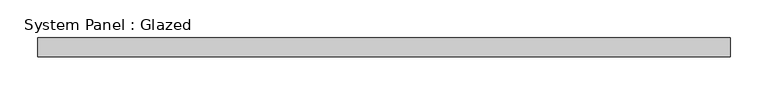
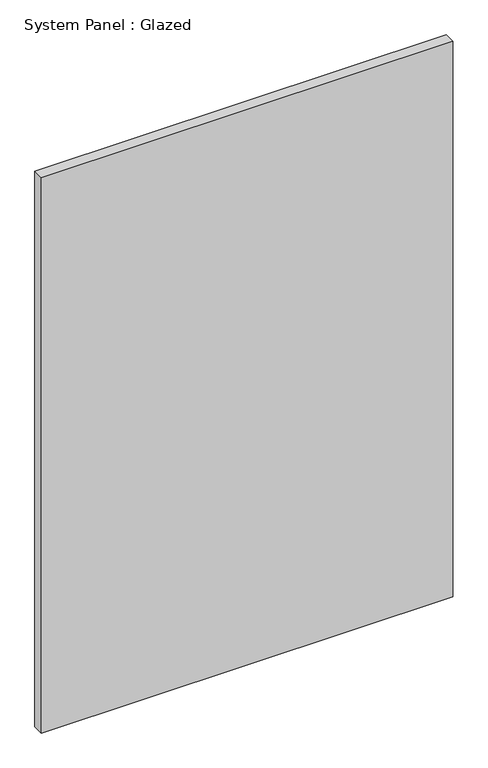
"""IFC4 building model written with IfcOpenShell, lengths in millimetres: plate geometry, System Panel : Glazed."""

from ifc_helpers import new_model, si_unit, origin, origin_with_axes, place, context, project, spatial, polyline, outline, extrude, source, transform, mapped, element, save


def system_panel_glazed_2f0fbb7d(model_context):
    return source(origin(), model_context, "Body", "SweptSolid", [
        extrude(outline(polyline([(460.375, 19.05), (-460.375, 19.05), (-460.375, 44.45), (460.375, 44.45), (460.375, 19.05)])), origin_with_axes(), (0.0, 0.0, 1.0), 1314.45),
    ])


if __name__ == "__main__":
    model = new_model("IFC4")
    model_context = context("Model", 3, world=origin())
    ifc_project = project(units=[si_unit("LENGTHUNIT", "METRE", prefix="MILLI")], contexts=[model_context])
    site = spatial("IfcSite", under=ifc_project)
    building = spatial("IfcBuilding", under=site)
    placement = place(None, origin())
    system_panel_glazed_shape = system_panel_glazed_2f0fbb7d(model_context)
    element("IfcPlate", 1, ObjectType="System Panel : Glazed", at=placement, inside=building, context=model_context, shape_type="MappedRepresentation", body=[
        mapped(system_panel_glazed_shape, transform((0.0, 0.0, 0.0), x_axis=(1.0, 0.0, 0.0), y_axis=(0.0, 1.0, 0.0), z_axis=(0.0, 0.0, 1.0))),
    ])
    save(model, "model.ifc")

# Revit data of these elements
# Type "System Panel : Glazed"
#   Construction Type Id = "GSP4R"
#   Analytic Construction = "1/8 in Pilkington single glazing"
#   Visual Light Transmittance = 0.9
#   Solar Heat Gain Coefficient = 0.86
#   Heat Transfer Coefficient (U) = 1.18115 BTU/(h·ft²·°F)
#   Define Thermal Properties by = 1
# Element 1 (IfcPlate, "System Panel : Glazed")
#   Materials on its faces: "Glass"
# Materials
#   "Glass": class "Glass", colour RGB 0 128 192, transparency 0.75, Description = "Soda Lime Glass", Cost = 0
